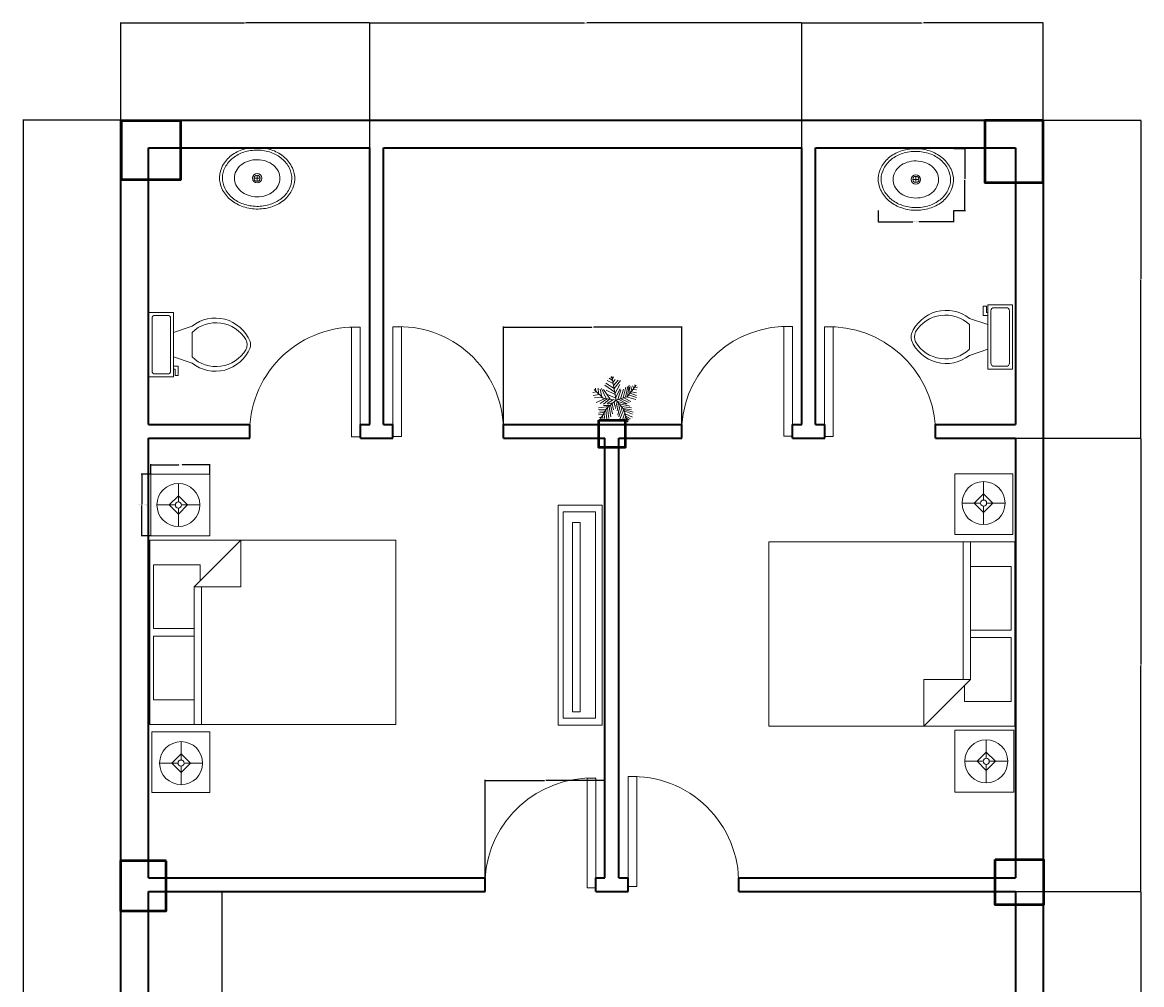
# Model space of a CAD drawing. Units: inches. Extents: x 50 to 2003, y -28 to 675.
# Tile 8 of 10: x 592 to 956, y 337 to 650. Entities that reach past the tile are written whole.
import ezdxf

# ---------------------------------------------------------------- set-up
doc = ezdxf.new("R2010")
doc.units = ezdxf.units.IN
for name, color, linetype, lineweight in [('A-ANNO-DIMS', 2, 'Continuous', 18), ('A-COLS', 1, 'Continuous', 50), ('A-DOOR', 4, 'Continuous', 18), ('A-FLOR-CASE', 32, 'Continuous', 25), ('A-FLOR-FIXT', 9, 'Continuous', 18), ('A-FURN', 8, 'Continuous', 18), ('A-FURN-LITE', 9, 'Continuous', 13), ('A-WALL', 7, 'Continuous', 35), ('L-PLNT', 3, 'Continuous', 13)]:
    doc.layers.add(name, color=color, linetype=linetype, lineweight=lineweight)
doc.styles.get("Standard").update_dxf_attribs({"font": 'arial.ttf'})
doc.dimstyles.get("Standard").update_dxf_attribs({"dimtxt": 0.18, "dimasz": 0.18, "dimexe": 0.18, "dimexo": 0.0625, "dimgap": 0.09, "dimtad": 0, "dimtih": 1, "dimtoh": 1, "dimdec": 4, "dimzin": 0, "dimdsep": 46, "dimtxsty": 'Standard', "dimcen": 0.09, "dimadec": 0, "dimazin": 0, "dimtfac": 1, "dimtdec": 4, "dimtofl": 0, "dimtmove": 0, "dimatfit": 3, "dimfxl": 1, "dimtolj": 1, "dimtzin": 0, "dimarcsym": 0})

# ---------------------------------------------------------------- blocks, each defined once
blk = doc.blocks.new('*U2')
for p, q in [((-10.186, 53.64), (-13.084, 55.962)), ((0, 0), (-10.5, 57)), ((-9.099, 51.782), (-6.563, 55.962)), ((-48.585, 21.131), (-49.309, 29.026)), ((-43.513, 28.561), (-42.427, 15.558)), ((-35.544, 28.097), (-24.314, 3.947)), ((-3.665, 19.273), (-27.574, 35.527)), ((-5.114, 28.097), (-24.676, 40.636)), ((-7.288, 39.707), (-21.778, 46.673)), ((-8.737, 47.138), (-17.069, 52.711)), ((-7.65, 43.423), (-2.578, 49.46)), ((-5.839, 35.992), (4.667, 48.067)), ((-5.114, 27.632), (10.463, 46.673)), ((-2.941, 16.486), (8.652, 37.85)), ((16.259, 5.805), (23.142, 31.348)), ((22.055, 7.198), (27.489, 32.277)), ((27, 9), (48, 36)), ((27.127, 9.056), (31.112, 35.992)), ((31.836, 30.883), (32.561, 16.486)), ((35.096, 32.741), (37.27, 22.524)), ((38.719, 34.134), (41.979, 28.561)), ((43.791, 29.954), (51.036, 30.883)), ((44.153, 36.456), (45.239, 32.741)), ((-47.498, 19.737), (-55.83, 18.344)), ((-40.615, 13.7), (-55.105, 10.913)), ((-31.5, 4.5), (-52.5, 25.5)), ((-33.37, 6.269), (-52.207, 5.34)), ((-28.299, 3.483), (-47.86, -5.805)), ((-38.442, 26.239), (-34.819, 7.663)), ((-21.416, 3.018), (-38.079, -8.128)), ((0, 0), (-31.5, 4.5)), ((-14.533, 2.09), (-30.834, 25.31)), ((-15.982, 2.09), (-30.11, -9.521)), ((-24.314, 23.917), (-2.941, 13.7)), ((0, 0), (-22.5, -19.5)), ((-6.563, 1.161), (-21.416, -8.128)), ((-20.691, 13.7), (-1.129, 4.876)), ((-1.129, 6.734), (9.014, 26.704)), ((0, 0), (27, 9)), ((0, 0), (18, -22.5)), ((3.942, 1.625), (11.187, 24.381)), ((6.478, 1.625), (26.04, -8.592)), ((10.101, 3.483), (17.708, 26.239)), ((11.187, 3.483), (30.749, -5.805)), ((18.07, 5.805), (35.096, -3.483)), ((24.229, 7.663), (46.688, 1.625)), ((29.662, 12.307), (48.137, 6.269)), ((33.285, 16.486), (48.862, 10.913)), ((36.183, 19.737), (48.137, 17.88)), ((40.53, 25.775), (48.862, 24.846)), ((-17.431, -15.094), (-42.789, -18.809)), ((-24.314, -21.596), (-42.427, -22.06)), ((-26.849, -26.24), (-40.253, -25.775)), ((-22.5, -19.5), (-37.5, -45)), ((-15.257, -12.772), (-30.11, -12.772)), ((-25.038, -23.918), (-22.865, -45.281)), ((-20.691, -18.345), (-17.793, -44.352)), ((-6.563, -5.805), (-19.967, -9.985)), ((-17.069, -15.094), (-12.721, -40.172)), ((-13.446, -11.378), (-8.737, -32.741)), ((-9.461, -8.592), (-6.201, -23.453)), ((-4.752, -3.483), (-3.665, -14.629)), ((2.493, -3.019), (-1.491, -20.202)), ((1.769, -2.555), (24.229, -9.521)), ((5.029, -6.27), (2.131, -25.775)), ((9.014, -11.378), (3.58, -35.992)), ((14.085, -16.951), (6.478, -40.172)), ((7.565, -9.056), (32.198, -14.629)), ((18.07, -22.524), (8.289, -45.745)), ((12.274, -15.094), (36.907, -18.809)), ((16.259, -19.738), (36.183, -22.989)), ((18, -22.5), (27, -52.5)), ((18.433, -22.524), (40.53, -29.026)), ((19.157, -25.311), (38.719, -33.206)), ((-28.299, -29.026), (-42.789, -31.348)), ((-30.834, -34.135), (-42.427, -35.528)), ((-34.457, -39.708), (-40.978, -42.494)), ((-32.646, -36.921), (-31.921, -44.352)), ((-29.023, -30.884), (-27.936, -43.887)), ((20.244, -30.419), (15.897, -44.816)), ((22.78, -37.85), (19.519, -48.532)), ((21.331, -32.741), (39.081, -40.636)), ((22.78, -38.314), (34.372, -44.816)), ((24.591, -45.745), (23.142, -50.854)), ((24.591, -43.423), (30.749, -47.603)), ((26.764, -49.925), (28.213, -50.854))]:
    blk.add_line(p, q)
blk = doc.blocks.new('Bed - Queen')
for p, q in [((0, -80.00003), (0, 0)), ((0, 0), (59.99999, 0)), ((59.99999, 0), (59.99999, -80.00003)), ((7.99999, -1.2), (28.79998, -1.2)), ((7.99999, -14.4), (7.99999, -1.2)), ((28.79998, -1.2), (28.79998, -14.4)), ((31.19999, -1.2), (51.99999, -1.2)), ((31.19999, -14.4), (31.19999, -1.2)), ((51.99999, -1.2), (51.99999, -16.4)), ((0, -14.4), (44.8, -14.4)), ((59.99999, -29.6), (44.8, -14.4)), ((44.8, -14.4), (44.8, -29.6)), ((44.8, -16.8), (0, -16.8)), ((51.99999, -16.4), (46.79936, -16.4)), ((44.8, -29.6), (59.99999, -29.6)), ((59.99999, -80.00003), (0, -80.00003))]:
    blk.add_line(p, q)
blk = doc.blocks.new('Lamp - Table')
for p, q in [((0, 7), (0, 1)), ((-1, 0), (-7, 0)), ((0, 3), (-3, 0)), ((-3, 0), (0, -3)), ((3, 0), (0, 3)), ((0, -3), (3, 0)), ((1, 0), (7, 0)), ((0, -1), (0, -7))]:
    blk.add_line(p, q)
for radius in [7, 1]:
    blk.add_circle((0, 0), radius)
blk = doc.blocks.new('Toilet - top')
for p, q in [((9.5, -6), (9.5, -2)), ((-10, -8.5), (-8, -8.5)), ((-10, -9.5), (-10, -8.5)), ((-7, -9.5), (-10, -9.5)), ((-8, -8.5), (-8, -8)), ((-7, -8), (-7, -9.5)), ((-4, -8), (-6, -14)), ((4, -8), (6, -14)), ((4, -14), (-4, -14))]:
    blk.add_line(p, q)
blk.add_lwpolyline([(10.5, -8), (10.5, 0), (-10.5, 0), (-10.5, -8)], close=True)
for points in [[(-9.5, -2), (-9.5, -6)], [(8.5, -1), (-8.5, -1)], [(-8.5, -7), (8.5, -7)]]:
    blk.add_lwpolyline(points)
for centre, radius, start, end in [((-8.62, -1.88), 0.884, 81.8699, 188.1301), ((8.62, -1.88), 0.884, 351.8699, 98.1301), ((-8.62, -6.12), 0.884, 171.8699, 278.1301), ((8.62, -6.12), 0.884, 261.8699, 8.1301), ((3.52, -21.58), 12.17, 141.4691, 247.9714), ((4.2, -21.82), 11.33, 136.3677, 238.9468), ((-3.52, -21.58), 12.17, 292.0284, 38.5307), ((-4.2, -21.82), 11.33, 301.053, 43.6321), ((0, -27.88), 4, 245.7318, 294.2682), ((0, -29), 4, 254.8605, 285.1395)]:
    blk.add_arc(centre, radius, start, end)
blk = doc.blocks.new('Sink - Oval top')
for p, q in [((-1, 0), (1, 0)), ((0, 1), (0, -1))]:
    blk.add_line(p, q)
for points in [[(-12.23, 0.39, 0.117634), (-11.46, -3.36, 0.104469), (-8.88, -6.8, 0.090016), (-5.08, -9.07, 0.08192), (-0.32, -10.02, 0.08192), (4.49, -9.38, 0.090016), (8.42, -7.36, 0.104469), (11.22, -4.09, 0.117634), (12.23, -0.39, 0.117634), (11.46, 3.36, 0.104469), (8.88, 6.8, 0.090016), (5.08, 9.07, 0.08192), (0.32, 10.02, 0.08192), (-4.49, 9.38, 0.090016), (-8.42, 7.36, 0.104469), (-11.22, 4.09, 0.117634)], [(-11.29, 0.16, 0.118622), (-10.52, -3.25, 0.104678), (-8.07, -6.36, 0.089562), (-4.54, -8.37, 0.081185), (-0.13, -9.15, 0.081185), (4.3, -8.49, 0.089562), (7.89, -6.58, 0.104678), (10.42, -3.55, 0.118622), (11.29, -0.16, 0.118622), (10.52, 3.25, 0.104678), (8.07, 6.36, 0.089562), (4.54, 8.37, 0.081185), (0.13, 9.15, 0.081185), (-4.3, 8.49, 0.089562), (-7.89, 6.58, 0.104678), (-10.42, 3.55, 0.118622)], [(-7.42, 0.08, 0.118283), (-6.91, -2.17, 0.104607), (-5.29, -4.21, 0.089718), (-2.97, -5.53, 0.081436), (-0.07, -6.04, 0.081436), (2.84, -5.59, 0.089718), (5.2, -4.33, 0.104607), (6.86, -2.32, 0.118283), (7.42, -0.08, 0.118283), (6.91, 2.17, 0.104607), (5.29, 4.21, 0.089718), (2.97, 5.53, 0.081436), (0.07, 6.04, 0.081436), (-2.84, 5.59, 0.089718), (-5.2, 4.33, 0.104607), (-6.86, 2.32, 0.118283)]]:
    blk.add_lwpolyline(points, format="xyb", close=True)
for radius in [1.5, 1]:
    blk.add_circle((0, 0), radius)
blk = doc.blocks.new('KITCHEN-COUNTER-L')
for q in [(0, 84), (54, 0)]:
    blk.add_line((0, 0), q)
blk = doc.blocks.new('MEDIA-CONSOLE')
for points in [[(0, 0), (71.49, 0), (71.49, 14.4), (0, 14.4)], [(2.13, 1.7), (69.3, 1.7), (69.3, 12.15), (2.13, 12.15)], [(5.56, 4.74), (67.2, 4.74), (67.2, 7.16), (5.56, 7.16)]]:
    blk.add_lwpolyline(points, close=True)
blk = doc.blocks.new('DOOR-LEAF-36')
blk.add_lwpolyline([(35.71, 2.81), (35.71, 0), (0, 0), (0, 2.81)], close=True)
blk = doc.blocks.new('NIGHTSTAND-COMPACT')
blk.add_lwpolyline([(0, 19.73), (0, 0), (18.92, 0), (18.92, 19.73)], close=True)
blk = doc.blocks.new('NIGHTSTAND-STANDARD')
blk.add_lwpolyline([(0, 0), (0, 20.13), (19.19, 20.13), (19.19, 0)], close=True)
blk = doc.blocks.new('*D27')
at = {"layer": 'A-ANNO-DIMS', "color": 0, "lineweight": -2, "transparency": 16777216}
for p, q in [((633.37, 503.48), (630.24, 503.48)), ((630.42, 503.3), (630.42, 493.59)), ((630.42, 483.52), (630.42, 493.23)), ((633.37, 483.34), (630.24, 483.34))]:
    blk.add_line(p, q, dxfattribs=at)
at = {"layer": 'A-ANNO-DIMS', "color": 0, "transparency": 16777216}
for points in [[(630.39, 503.3), (630.45, 503.3), (630.42, 503.48)], [(630.39, 483.52), (630.45, 483.52), (630.42, 483.34)]]:
    blk.add_solid(points, dxfattribs=at)
at = {"layer": 'Defpoints', "color": 0, "transparency": 16777216}
for p in [(630.42, 503.48), (633.44, 503.48), (633.44, 483.34)]:
    blk.add_point(p, dxfattribs=at)
at = {"layer": 'A-ANNO-DIMS', "color": 0, "transparency": 16777216, "insert": (630.42, 493.41), "char_height": 0.18, "attachment_point": 5}
blk.add_mtext('\\A1;STANDARD NIGHTSTAND 20 TYP.', dxfattribs=at)
blk = doc.blocks.new('*D28')
at = {"layer": 'A-ANNO-DIMS', "color": 0, "lineweight": -2, "transparency": 16777216}
for p, q in [((633.44, 503.54), (633.44, 506.68)), ((633.62, 506.5), (642.51, 506.5)), ((652.44, 506.5), (643.55, 506.5)), ((652.62, 503.54), (652.62, 506.68))]:
    blk.add_line(p, q, dxfattribs=at)
at = {"layer": 'A-ANNO-DIMS', "color": 0, "transparency": 16777216}
for points in [[(633.62, 506.53), (633.62, 506.47), (633.44, 506.5)], [(652.44, 506.53), (652.44, 506.47), (652.62, 506.5)]]:
    blk.add_solid(points, dxfattribs=at)
at = {"layer": 'Defpoints', "color": 0, "transparency": 16777216}
for p in [(652.62, 506.5), (633.44, 503.48), (652.62, 503.48)]:
    blk.add_point(p, dxfattribs=at)
at = {"layer": 'A-ANNO-DIMS', "color": 0, "transparency": 16777216, "insert": (643.03, 506.5), "char_height": 0.18, "attachment_point": 5}
blk.add_mtext('\\A1;19 TYP.', dxfattribs=at)
blk = doc.blocks.new('*D31')
at = {"layer": 'A-ANNO-DIMS', "color": 0, "lineweight": -2, "transparency": 16777216}
for p, q in [((869.97, 589.2), (869.97, 585.4)), ((894.52, 589.2), (894.52, 585.4)), ((870.15, 585.58), (881.31, 585.58)), ((894.34, 585.58), (883.18, 585.58))]:
    blk.add_line(p, q, dxfattribs=at)
at = {"layer": 'A-ANNO-DIMS', "color": 0, "transparency": 16777216}
for points in [[(870.15, 585.61), (870.15, 585.55), (869.97, 585.58)], [(894.34, 585.61), (894.34, 585.55), (894.52, 585.58)]]:
    blk.add_solid(points, dxfattribs=at)
at = {"layer": 'Defpoints', "color": 0, "transparency": 16777216}
for p in [(869.97, 589.26), (894.52, 589.26), (894.52, 585.58)]:
    blk.add_point(p, dxfattribs=at)
at = {"layer": 'A-ANNO-DIMS', "color": 0, "transparency": 16777216, "insert": (882.24, 585.58), "char_height": 0.18, "attachment_point": 5}
blk.add_mtext('\\A1;BASIN 25 TYP.', dxfattribs=at)
blk = doc.blocks.new('*D32')
at = {"layer": 'A-ANNO-DIMS', "color": 0, "lineweight": -2, "transparency": 16777216}
for p, q in [((894.58, 609.4), (898.38, 609.4)), ((898.2, 609.22), (898.2, 599.51)), ((898.2, 589.44), (898.2, 599.15)), ((894.58, 589.26), (898.38, 589.26))]:
    blk.add_line(p, q, dxfattribs=at)
at = {"layer": 'A-ANNO-DIMS', "color": 0, "transparency": 16777216}
for points in [[(898.17, 609.22), (898.23, 609.22), (898.2, 609.4)], [(898.17, 589.44), (898.23, 589.44), (898.2, 589.26)]]:
    blk.add_solid(points, dxfattribs=at)
at = {"layer": 'Defpoints', "color": 0, "transparency": 16777216}
for p in [(894.52, 609.4), (898.2, 609.4), (894.52, 589.26)]:
    blk.add_point(p, dxfattribs=at)
at = {"layer": 'A-ANNO-DIMS', "color": 0, "transparency": 16777216, "insert": (898.2, 599.33), "char_height": 0.18, "attachment_point": 5}
blk.add_mtext('\\A1;20 TYP.', dxfattribs=at)
blk = doc.blocks.new('*D75')
at = {"layer": 'A-ANNO-DIMS', "color": 0, "lineweight": -2, "transparency": 16777216}
for p, q in [((623.55, 618.62), (591.74, 618.62)), ((591.92, 618.44), (591.92, 311.25)), ((591.92, 3.7), (591.92, 310.89)), ((623.59, 3.52), (591.74, 3.52))]:
    blk.add_line(p, q, dxfattribs=at)
at = {"layer": 'A-ANNO-DIMS', "color": 0, "transparency": 16777216}
for points in [[(591.89, 618.44), (591.95, 618.44), (591.92, 618.62)], [(591.89, 3.7), (591.95, 3.7), (591.92, 3.52)]]:
    blk.add_solid(points, dxfattribs=at)
at = {"layer": 'Defpoints', "color": 0, "transparency": 16777216}
for p in [(591.92, 618.62), (623.62, 618.62), (623.65, 3.52)]:
    blk.add_point(p, dxfattribs=at)
at = {"layer": 'A-ANNO-DIMS', "color": 0, "transparency": 16777216, "insert": (591.92, 311.07), "char_height": 0.18, "attachment_point": 5}
blk.add_mtext('\\A1;615.1', dxfattribs=at)
blk = doc.blocks.new('*D77')
at = {"layer": 'A-ANNO-DIMS', "color": 0, "lineweight": -2, "transparency": 16777216}
for p, q in [((623.62, 618.68), (623.62, 650.45)), ((623.8, 650.27), (663.91, 650.27)), ((704.44, 650.27), (664.32, 650.27)), ((704.62, 609.68), (704.62, 650.45))]:
    blk.add_line(p, q, dxfattribs=at)
at = {"layer": 'A-ANNO-DIMS', "color": 0, "transparency": 16777216}
for points in [[(623.8, 650.3), (623.8, 650.24), (623.62, 650.27)], [(704.44, 650.3), (704.44, 650.24), (704.62, 650.27)]]:
    blk.add_solid(points, dxfattribs=at)
at = {"layer": 'Defpoints', "color": 0, "transparency": 16777216}
for p in [(704.62, 650.27), (623.62, 618.62), (704.62, 609.62)]:
    blk.add_point(p, dxfattribs=at)
at = {"layer": 'A-ANNO-DIMS', "color": 0, "transparency": 16777216, "insert": (664.12, 650.27), "char_height": 0.18, "attachment_point": 5}
blk.add_mtext('\\A1;81', dxfattribs=at)
blk = doc.blocks.new('*D78')
at = {"layer": 'A-ANNO-DIMS', "color": 0, "lineweight": -2, "transparency": 16777216}
for p, q in [((704.62, 609.68), (704.62, 650.45)), ((704.8, 650.27), (774.48, 650.27)), ((844.94, 650.27), (775.25, 650.27)), ((845.12, 609.68), (845.12, 650.45))]:
    blk.add_line(p, q, dxfattribs=at)
at = {"layer": 'A-ANNO-DIMS', "color": 0, "transparency": 16777216}
for points in [[(704.8, 650.3), (704.8, 650.24), (704.62, 650.27)], [(844.94, 650.3), (844.94, 650.24), (845.12, 650.27)]]:
    blk.add_solid(points, dxfattribs=at)
at = {"layer": 'Defpoints', "color": 0, "transparency": 16777216}
for p in [(845.12, 650.27), (704.62, 609.62), (845.12, 609.62)]:
    blk.add_point(p, dxfattribs=at)
at = {"layer": 'A-ANNO-DIMS', "color": 0, "transparency": 16777216, "insert": (774.87, 650.27), "char_height": 0.18, "attachment_point": 5}
blk.add_mtext('\\A1;140.5', dxfattribs=at)
blk = doc.blocks.new('*D79')
at = {"layer": 'A-ANNO-DIMS', "color": 0, "lineweight": -2, "transparency": 16777216}
for p, q in [((845.12, 609.68), (845.12, 650.45)), ((845.3, 650.27), (884.04, 650.27)), ((923.44, 650.27), (884.69, 650.27)), ((923.62, 618.68), (923.62, 650.45))]:
    blk.add_line(p, q, dxfattribs=at)
at = {"layer": 'A-ANNO-DIMS', "color": 0, "transparency": 16777216}
for points in [[(845.3, 650.3), (845.3, 650.24), (845.12, 650.27)], [(923.44, 650.3), (923.44, 650.24), (923.62, 650.27)]]:
    blk.add_solid(points, dxfattribs=at)
at = {"layer": 'Defpoints', "color": 0, "transparency": 16777216}
for p in [(923.62, 650.27), (923.62, 618.62), (845.12, 609.62)]:
    blk.add_point(p, dxfattribs=at)
at = {"layer": 'A-ANNO-DIMS', "color": 0, "transparency": 16777216, "insert": (884.37, 650.27), "char_height": 0.18, "attachment_point": 5}
blk.add_mtext('\\A1;78.5', dxfattribs=at)
blk = doc.blocks.new('*D82')
at = {"layer": 'A-ANNO-DIMS', "color": 0, "lineweight": -2, "transparency": 16777216}
for p, q in [((914.68, 367.62), (955.56, 367.62)), ((955.38, 367.44), (955.38, 283.55)), ((955.38, 199.3), (955.38, 283.19)), ((914.68, 199.12), (955.56, 199.12))]:
    blk.add_line(p, q, dxfattribs=at)
at = {"layer": 'A-ANNO-DIMS', "color": 0, "transparency": 16777216}
for points in [[(955.35, 367.44), (955.41, 367.44), (955.38, 367.62)], [(955.35, 199.3), (955.41, 199.3), (955.38, 199.12)]]:
    blk.add_solid(points, dxfattribs=at)
at = {"layer": 'Defpoints', "color": 0, "transparency": 16777216}
for p in [(914.62, 367.62), (955.38, 367.62), (914.62, 199.12)]:
    blk.add_point(p, dxfattribs=at)
at = {"layer": 'A-ANNO-DIMS', "color": 0, "transparency": 16777216, "insert": (955.38, 283.37), "char_height": 0.18, "attachment_point": 5}
blk.add_mtext('\\A1;168.5', dxfattribs=at)
blk = doc.blocks.new('*D83')
at = {"layer": 'A-ANNO-DIMS', "color": 0, "lineweight": -2, "transparency": 16777216}
for p, q in [((914.68, 515.12), (955.56, 515.12)), ((955.38, 514.94), (955.38, 441.55)), ((955.38, 367.8), (955.38, 441.19)), ((914.68, 367.62), (955.56, 367.62))]:
    blk.add_line(p, q, dxfattribs=at)
at = {"layer": 'A-ANNO-DIMS', "color": 0, "transparency": 16777216}
for points in [[(955.35, 514.94), (955.41, 514.94), (955.38, 515.12)], [(955.35, 367.8), (955.41, 367.8), (955.38, 367.62)]]:
    blk.add_solid(points, dxfattribs=at)
at = {"layer": 'Defpoints', "color": 0, "transparency": 16777216}
for p in [(914.62, 515.12), (955.38, 515.12), (914.62, 367.62)]:
    blk.add_point(p, dxfattribs=at)
at = {"layer": 'A-ANNO-DIMS', "color": 0, "transparency": 16777216, "insert": (955.38, 441.37), "char_height": 0.18, "attachment_point": 5}
blk.add_mtext('\\A1;147.5', dxfattribs=at)
blk = doc.blocks.new('*D84')
at = {"layer": 'A-ANNO-DIMS', "color": 0, "lineweight": -2, "transparency": 16777216}
for p, q in [((923.68, 618.62), (955.56, 618.62)), ((955.38, 618.44), (955.38, 567.05)), ((955.38, 515.3), (955.38, 566.69)), ((914.68, 515.12), (955.56, 515.12))]:
    blk.add_line(p, q, dxfattribs=at)
at = {"layer": 'A-ANNO-DIMS', "color": 0, "transparency": 16777216}
for points in [[(955.35, 618.44), (955.41, 618.44), (955.38, 618.62)], [(955.35, 515.3), (955.41, 515.3), (955.38, 515.12)]]:
    blk.add_solid(points, dxfattribs=at)
at = {"layer": 'Defpoints', "color": 0, "transparency": 16777216}
for p in [(923.62, 618.62), (955.38, 618.62), (914.62, 515.12)]:
    blk.add_point(p, dxfattribs=at)
at = {"layer": 'A-ANNO-DIMS', "color": 0, "transparency": 16777216, "insert": (955.38, 566.87), "char_height": 0.18, "attachment_point": 5}
blk.add_mtext('\\A1;103.5', dxfattribs=at)
blk = doc.blocks.new('*D92')
at = {"layer": 'A-ANNO-DIMS', "color": 0, "lineweight": -2, "transparency": 16777216}
for p, q in [((748.12, 519.68), (748.12, 551.45)), ((748.3, 551.27), (776.9, 551.27)), ((805.94, 551.27), (777.34, 551.27)), ((806.12, 519.68), (806.12, 551.45))]:
    blk.add_line(p, q, dxfattribs=at)
at = {"layer": 'A-ANNO-DIMS', "color": 0, "transparency": 16777216}
for points in [[(748.3, 551.3), (748.3, 551.24), (748.12, 551.27)], [(805.94, 551.3), (805.94, 551.24), (806.12, 551.27)]]:
    blk.add_solid(points, dxfattribs=at)
at = {"layer": 'Defpoints', "color": 0, "transparency": 16777216}
for p in [(806.12, 551.27), (748.12, 519.62), (806.12, 519.62)]:
    blk.add_point(p, dxfattribs=at)
at = {"layer": 'A-ANNO-DIMS', "color": 0, "transparency": 16777216, "insert": (777.12, 551.27), "char_height": 0.18, "attachment_point": 5}
blk.add_mtext('\\A1;58', dxfattribs=at)
blk = doc.blocks.new('*D93')
at = {"layer": 'A-ANNO-DIMS', "color": 0, "lineweight": -2, "transparency": 16777216}
for p, q in [((742.12, 372.18), (742.12, 403.95)), ((742.3, 403.77), (761.4, 403.77)), ((780.94, 403.77), (761.84, 403.77)), ((781.12, 372.18), (781.12, 403.95))]:
    blk.add_line(p, q, dxfattribs=at)
at = {"layer": 'A-ANNO-DIMS', "color": 0, "transparency": 16777216}
for points in [[(742.3, 403.8), (742.3, 403.74), (742.12, 403.77)], [(780.94, 403.8), (780.94, 403.74), (781.12, 403.77)]]:
    blk.add_solid(points, dxfattribs=at)
at = {"layer": 'Defpoints', "color": 0, "transparency": 16777216}
for p in [(781.12, 403.77), (742.12, 372.12), (781.12, 372.12)]:
    blk.add_point(p, dxfattribs=at)
at = {"layer": 'A-ANNO-DIMS', "color": 0, "transparency": 16777216, "insert": (761.62, 403.77), "char_height": 0.18, "attachment_point": 5}
blk.add_mtext('\\A1;39', dxfattribs=at)

msp = doc.modelspace()

# ---------------------------------------------------------------- linework, layer by layer
at = {"layer": 'A-COLS'}
for points in [[(623.8056, 618.497), (643.0413, 618.497), (643.0413, 599.2734), (623.8056, 599.2734)], [(923.6503, 618.4953), (904.7316, 618.4953), (904.7316, 598.4027), (923.6503, 598.4027)], [(779.1289, 521.0096), (787.6835, 521.0096), (787.6835, 512.1331), (779.1289, 512.1331)], [(638.3683, 377.5957), (623.5732, 377.5957), (623.5732, 361.3313), (638.3683, 361.3313)], [(908.101, 378.1167), (923.7293, 378.1167), (923.7293, 363.3442), (908.101, 363.3442)]]:
    msp.add_lwpolyline(points, close=True, dxfattribs=at)
at = {"layer": 'A-DOOR'}
for centre, radius, start, end in [((699.7556, 517.099), 34.1945, 87.058708, 178.785816), ((714.2004, 517.539), 33.9127, 1.649886, 93.532481), ((840.5394, 517.0208), 34.5264, 87.442535, 175.833183), ((853.9486, 516.6707), 34.7564, 3.698129, 92.267605), ((776.9185, 369.747), 34.8827, 88.052675, 176.477707), ((790.0974, 370.563), 34.5082, 358.96058, 92.308257)]:
    msp.add_arc(centre, radius, start, end, dxfattribs=at)
at = {"layer": 'A-WALL'}
for p, q in [((623.6163, 3.6217), (623.6163, 618.6217)), ((623.6163, 618.6217), (923.6163, 618.6217)), ((923.6163, 618.6217), (923.6163, 3.6217)), ((632.6163, 609.6217), (704.6163, 609.6217)), ((632.6163, 519.6217), (632.6163, 609.6217)), ((704.6163, 519.6217), (704.6163, 609.6217)), ((709.1163, 519.6217), (709.1163, 609.6217)), ((709.1163, 609.6217), (845.1163, 609.6217)), ((845.1163, 519.6217), (845.1163, 609.6217)), ((849.6163, 519.6217), (849.6163, 609.6217)), ((849.6163, 609.6217), (914.6163, 609.6217)), ((914.6163, 609.6217), (914.6163, 519.6217)), ((632.6163, 519.6217), (665.6163, 519.6217)), ((665.6163, 515.1217), (665.6163, 519.6217)), ((701.6163, 515.1217), (701.6163, 519.6217)), ((701.6163, 519.6217), (704.6163, 519.6217)), ((709.1163, 519.6217), (712.1163, 519.6217)), ((712.1163, 515.1217), (712.1163, 519.6217)), ((748.1163, 515.1217), (748.1163, 519.6217)), ((748.1163, 519.6217), (806.1163, 519.6217)), ((806.1163, 515.1217), (806.1163, 519.6217)), ((842.1163, 515.1217), (842.1163, 519.6217)), ((842.1163, 519.6217), (845.1163, 519.6217)), ((849.6163, 519.6217), (852.6163, 519.6217)), ((852.6163, 515.1217), (852.6163, 519.6217)), ((888.6163, 515.1217), (888.6163, 519.6217)), ((888.6163, 519.6217), (914.6163, 519.6217)), ((632.6163, 515.1217), (665.6163, 515.1217)), ((632.6163, 372.1216), (632.6163, 515.1217)), ((701.6163, 515.1217), (712.1163, 515.1217)), ((748.1163, 515.1217), (781.1163, 515.1217)), ((781.1163, 372.1216), (781.1163, 515.1217)), ((785.6163, 372.1216), (785.6163, 515.1217)), ((785.6163, 515.1217), (806.1163, 515.1217)), ((842.1163, 515.1217), (852.6163, 515.1217)), ((888.6163, 515.1217), (914.6163, 515.1217)), ((914.6163, 515.1217), (914.6163, 372.1216)), ((632.6163, 372.1216), (742.1163, 372.1216)), ((742.1163, 367.6216), (742.1163, 372.1216)), ((778.1163, 367.6216), (778.1163, 372.1216)), ((778.1163, 372.1216), (781.1163, 372.1216)), ((785.6163, 372.1216), (788.6163, 372.1216)), ((788.6163, 367.6216), (788.6163, 372.1216)), ((824.6163, 367.6216), (824.6163, 372.1216)), ((824.6163, 372.1216), (914.6163, 372.1216)), ((632.6163, 367.6216), (742.1163, 367.6216)), ((632.6163, 259.6217), (632.6163, 367.6216)), ((778.1163, 367.6216), (788.6163, 367.6216)), ((824.6163, 367.6216), (914.6163, 367.6216)), ((914.6163, 367.6216), (914.6163, 203.6217))]:
    msp.add_line(p, q, dxfattribs=at)

# ---------------------------------------------------------------- block references
at = {"layer": 'A-DOOR', "rotation": 269.9999999999999}
for p in [(698.7262, 551.3016), (712.0863, 551.4232), (839.2935, 551.5286), (852.5694, 551.4004), (775.3113, 404.5964), (788.6522, 405.0408)]:
    msp.add_blockref('DOOR-LEAF-36', p, dxfattribs=at)
at = {"layer": 'A-FLOR-CASE'}
msp.add_blockref('KITCHEN-COUNTER-L', (656.6163, 283.6217), dxfattribs=at)
at = {"layer": 'A-FLOR-FIXT'}
for p in [(667.9835, 599.7409), (882.2436, 599.3327)]:
    msp.add_blockref('Sink - Oval top', p, dxfattribs=at)
for p, rotation in [((913.6775, 548.104), 270), ((632.8007, 545.595), 89.99999999999999)]:
    msp.add_blockref('Toilet - top', p, dxfattribs=dict(at, rotation=rotation))
at = {"layer": 'A-FURN'}
for name, p in [('NIGHTSTAND-STANDARD', (633.4352, 483.3416)), ('NIGHTSTAND-COMPACT', (633.7017, 399.8715))]:
    msp.add_blockref(name, p, dxfattribs=at)
for name, p, rotation in [('NIGHTSTAND-COMPACT', (913.8149, 503.5813), 180), ('MEDIA-CONSOLE', (765.8633, 493.3173), 269.9999999999994), ('Bed - Queen', (633.0415, 421.9879), 90), ('Bed - Queen', (914.4752, 481.4648), 270), ('NIGHTSTAND-STANDARD', (914.0814, 420.1112), 180)]:
    msp.add_blockref(name, p, dxfattribs=dict(at, rotation=rotation))
at = {"layer": 'A-FURN-LITE'}
for p, rotation in [((642.3769, 493.4236), 90), ((904.2667, 494.0269), 270), ((643.2499, 409.4258), 90), ((905.1398, 410.0291), 270)]:
    msp.add_blockref('Lamp - Table', p, dxfattribs=dict(at, rotation=rotation))
at = {"layer": 'L-PLNT', "xscale": 0.1358686367750108, "yscale": 0.1358686367750108, "zscale": 0.1358686367750108}
msp.add_blockref('*U2', (784.7882, 527.5407), dxfattribs=at)

# ---------------------------------------------------------------- dimensions: what is measured, and where the dimension line sits
at = {"layer": 'A-ANNO-DIMS'}
for base, p1, p2, override, picture, middle in [((704.6163, 650.2717), (623.6163, 618.6217), (704.6163, 609.6217), {"dimdec": 0, "dimlfac": 1, "dimrnd": 0, "dimzin": 0, "dimdsep": 46, "dimlunit": 2}, '*D77', (664.1163, 650.2717)), ((845.1163, 650.2717), (704.6163, 609.6217), (845.1163, 609.6217), {"dimdec": 1, "dimlfac": 1, "dimrnd": 0, "dimzin": 0, "dimdsep": 46, "dimlunit": 2}, '*D78', (774.8663, 650.2717)), ((923.6163, 650.2717), (845.1163, 609.6217), (923.6163, 618.6217), {"dimdec": 1, "dimlfac": 1, "dimrnd": 0, "dimzin": 0, "dimdsep": 46, "dimlunit": 2}, '*D79', (884.3663, 650.2717)), ((806.1163, 551.2717), (748.1163, 519.6217), (806.1163, 519.6217), {"dimdec": 0, "dimlfac": 1, "dimrnd": 0, "dimzin": 0, "dimdsep": 46, "dimlunit": 2}, '*D92', (777.1163, 551.2717))]:
    dim = msp.add_linear_dim(base=base, p1=p1, p2=p2, dimstyle='Standard', override=override, dxfattribs=at)
    dim.commit()
    dim.dimension.update_dxf_attribs({"geometry": picture, "text_midpoint": middle})
for base, p1, p2, angle, override, picture, middle in [((591.9232, 618.6217), (623.6536, 3.5196), (623.6163, 618.6217), 90, {"dimdec": 1, "dimlfac": 1, "dimrnd": 0, "dimzin": 0, "dimdsep": 46, "dimlunit": 2}, '*D75', (591.9232, 311.0706)), ((955.3793, 618.6217), (914.6163, 515.1217), (923.6163, 618.6217), 90, {"dimdec": 1, "dimlfac": 1, "dimrnd": 0, "dimzin": 0, "dimdsep": 46, "dimlunit": 2}, '*D84', (955.3793, 566.8716)), ((955.3793, 515.1217), (914.6163, 367.6216), (914.6163, 515.1217), 90, {"dimdec": 1, "dimlfac": 1, "dimrnd": 0, "dimzin": 0, "dimdsep": 46, "dimlunit": 2}, '*D83', (955.3793, 441.3716)), ((781.1163, 403.7717), (742.1163, 372.1216), (781.1163, 372.1216), 0, {"dimdec": 0, "dimlfac": 1, "dimrnd": 0, "dimzin": 0, "dimdsep": 46, "dimlunit": 2}, '*D93', (761.6163, 403.7717)), ((955.3793, 367.6216), (914.6163, 199.1216), (914.6163, 367.6216), 90, {"dimdec": 1, "dimlfac": 1, "dimrnd": 0, "dimzin": 0, "dimdsep": 46, "dimlunit": 2}, '*D82', (955.3793, 283.3716))]:
    dim = msp.add_linear_dim(base=base, p1=p1, p2=p2, angle=angle, dimstyle='Standard', override=override, dxfattribs=at)
    dim.commit()
    dim.dimension.update_dxf_attribs({"geometry": picture, "text_midpoint": middle})
for base, p1, p2, text, picture, middle in [((898.2017, 609.401), (894.519, 589.2644), (894.519, 609.401), '<> TYP.', '*D32', (898.2017, 599.3327)), ((630.4151, 503.4757), (633.4352, 483.3416), (633.4352, 503.4757), 'STANDARD NIGHTSTAND <> TYP.', '*D27', (630.4151, 493.4087))]:
    dim = msp.add_linear_dim(base=base, p1=p1, p2=p2, angle=90, text=text, dimstyle='Standard', override={"dimdec": 0, "dimlfac": 1, "dimrnd": 0, "dimzin": 0, "dimdsep": 46, "dimlunit": 2}, dxfattribs=at)
    dim.commit()
    dim.dimension.update_dxf_attribs({"geometry": picture, "text_midpoint": middle})
for base, p1, p2, text, picture, middle in [((894.519, 585.5817), (869.9682, 589.2644), (894.519, 589.2644), 'BASIN <> TYP.', '*D31', (882.2436, 585.5817)), ((652.624, 506.4959), (633.4352, 503.4757), (652.624, 503.4757), '<> TYP.', '*D28', (643.0296, 506.4959))]:
    dim = msp.add_linear_dim(base=base, p1=p1, p2=p2, text=text, dimstyle='Standard', override={"dimdec": 0, "dimlfac": 1, "dimrnd": 0, "dimzin": 0, "dimdsep": 46, "dimlunit": 2}, dxfattribs=at)
    dim.commit()
    dim.dimension.update_dxf_attribs({"geometry": picture, "text_midpoint": middle})

doc.saveas('drawing.dxf')
